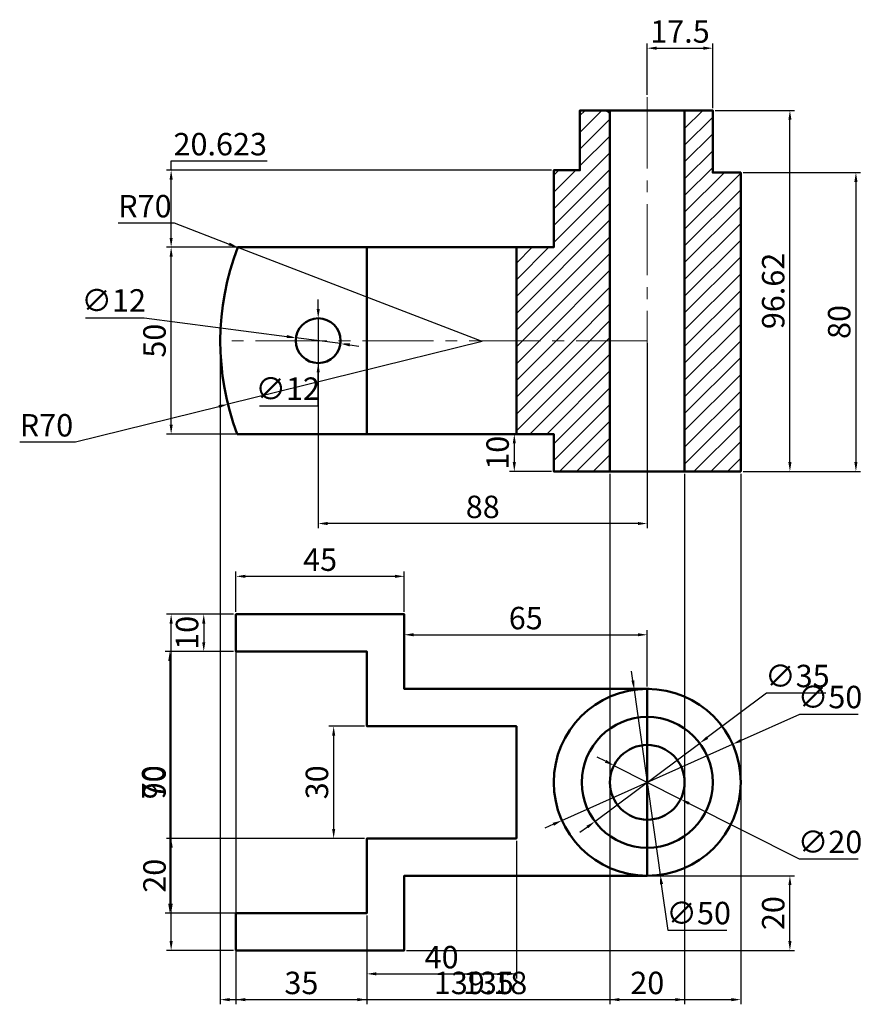
# Model space of a CAD drawing. Units: millimetres. Extents: x -19 to 206, y 5 to 269.
import ezdxf

# ---------------------------------------------------------------- set-up
doc = ezdxf.new("R2010")
doc.units = ezdxf.units.MM
doc.linetypes.add('CENTER2', pattern=[28.575, 19.05, -3.175, 3.175, -3.175])
for name, color, linetype, lineweight in [('M-CNTR', 4, 'CENTER2', 18), ('M-DIMS', 2, 'Continuous', 25), ('M-HATC', 8, 'Continuous', 18), ('M-OUTL', 7, 'Continuous', 50)]:
    doc.layers.add(name, color=color, linetype=linetype, lineweight=lineweight)
doc.styles.get("Standard").update_dxf_attribs({"font": 'arial.ttf'})
doc.dimstyles.new('ISO-25', dxfattribs={"dimtxt": 6, "dimasz": 2.5, "dimexe": 1.25, "dimexo": 0.625, "dimtad": 1, "dimtoh": 1, "dimdec": 0, "dimtxsty": 'Standard', "dimcen": 2.5, "dimadec": 0, "dimazin": 0, "dimtfac": 1, "dimtdec": 0, "dimtmove": 0, "dimatfit": 3, "dimfxl": 1, "dimarcsym": 0})

# ---------------------------------------------------------------- blocks, each defined once
blk = doc.blocks.new('*D1')
at = {"layer": 'Defpoints', "color": 0, "transparency": 16777216}
for p in [(54.94, 183.69), (66.84, 182.12)]:
    blk.add_point(p, dxfattribs=at)
at = {"layer": 'M-DIMS', "color": 0, "lineweight": -2, "transparency": 16777216}
for p, q in [((-1.34, 189.05), (14.35, 189.05)), ((14.35, 189.05), (52.46, 184.02)), ((66.84, 182.12), (54.94, 183.69)), ((69.31, 181.8), (71.79, 181.47))]:
    blk.add_line(p, q, dxfattribs=at)
at = {"layer": 'M-DIMS', "color": 0, "transparency": 16777216}
for points in [[(52.52, 184.43), (52.41, 183.61), (54.94, 183.69)], [(69.37, 182.21), (69.26, 181.38), (66.84, 182.12)]]:
    blk.add_solid(points, dxfattribs=at)
at = {"layer": 'M-DIMS', "color": 0, "transparency": 16777216, "insert": (6.19, 192.91), "char_height": 6, "attachment_point": 5}
blk.add_mtext('∅12', dxfattribs=at)
blk = doc.blocks.new('*D2')
at = {"layer": 'Defpoints', "color": 0, "transparency": 16777216}
for p in [(39.38, 207.88), (104.7, 182.73)]:
    blk.add_point(p, dxfattribs=at)
at = {"layer": 'M-DIMS', "color": 0, "lineweight": -2, "transparency": 16777216}
for p, q in [((7.38, 214.44), (22.32, 214.44)), ((22.32, 214.44), (37.04, 208.78)), ((104.7, 182.73), (39.38, 207.88))]:
    blk.add_line(p, q, dxfattribs=at)
at = {"layer": 'M-DIMS', "color": 0, "transparency": 16777216}
blk.add_solid([(37.19, 209.17), (36.89, 208.39), (39.38, 207.88)], dxfattribs=at)
at = {"layer": 'M-DIMS', "color": 0, "transparency": 16777216, "insert": (14.54, 218.13), "char_height": 6, "attachment_point": 5}
blk.add_mtext('R70', dxfattribs=at)
blk = doc.blocks.new('*D3')
at = {"layer": 'Defpoints', "color": 0, "transparency": 16777216}
for p in [(173.89, 227.91), (173.89, 147.91), (204.69, 147.91)]:
    blk.add_point(p, dxfattribs=at)
at = {"layer": 'M-DIMS', "color": 0, "lineweight": -2, "transparency": 16777216}
for p, q in [((174.51, 227.91), (205.94, 227.91)), ((204.69, 225.41), (204.69, 150.41)), ((174.51, 147.91), (205.94, 147.91))]:
    blk.add_line(p, q, dxfattribs=at)
at = {"layer": 'M-DIMS', "color": 0, "transparency": 16777216}
for points in [[(204.27, 225.41), (205.1, 225.41), (204.69, 227.91)], [(204.27, 150.41), (205.1, 150.41), (204.69, 147.91)]]:
    blk.add_solid(points, dxfattribs=at)
at = {"layer": 'M-DIMS', "color": 0, "transparency": 16777216, "insert": (201, 187.91), "char_height": 6, "attachment_point": 5, "rotation": 90}
blk.add_mtext('80', dxfattribs=at)
blk = doc.blocks.new('*D4')
at = {"layer": 'Defpoints', "color": 0, "transparency": 16777216}
for p in [(123.89, 157.91), (113.33, 147.91), (123.89, 147.91)]:
    blk.add_point(p, dxfattribs=at)
at = {"layer": 'M-DIMS', "color": 0, "lineweight": -2, "transparency": 16777216}
for p, q in [((123.26, 157.91), (112.08, 157.91)), ((113.33, 155.41), (113.33, 150.41)), ((123.26, 147.91), (112.08, 147.91))]:
    blk.add_line(p, q, dxfattribs=at)
at = {"layer": 'M-DIMS', "color": 0, "transparency": 16777216}
for points in [[(112.91, 155.41), (113.74, 155.41), (113.33, 157.91)], [(112.91, 150.41), (113.74, 150.41), (113.33, 147.91)]]:
    blk.add_solid(points, dxfattribs=at)
at = {"layer": 'M-DIMS', "color": 0, "transparency": 16777216, "insert": (109.64, 152.91), "char_height": 6, "attachment_point": 5, "rotation": 90}
blk.add_mtext('10', dxfattribs=at)
blk = doc.blocks.new('*D5')
at = {"layer": 'Defpoints', "color": 0, "transparency": 16777216}
for p in [(60.89, 182.91), (148.89, 182.91), (60.89, 133.98)]:
    blk.add_point(p, dxfattribs=at)
at = {"layer": 'M-DIMS', "color": 0, "lineweight": -2, "transparency": 16777216}
for p, q in [((60.89, 182.28), (60.89, 132.73)), ((148.89, 182.28), (148.89, 132.73)), ((146.39, 133.98), (63.39, 133.98))]:
    blk.add_line(p, q, dxfattribs=at)
at = {"layer": 'M-DIMS', "color": 0, "transparency": 16777216}
for points in [[(63.39, 134.39), (63.39, 133.56), (60.89, 133.98)], [(146.39, 134.39), (146.39, 133.56), (148.89, 133.98)]]:
    blk.add_solid(points, dxfattribs=at)
at = {"layer": 'M-DIMS', "color": 0, "transparency": 16777216, "insert": (104.89, 137.66), "char_height": 6, "attachment_point": 5}
blk.add_mtext('88', dxfattribs=at)
blk = doc.blocks.new('*D6')
at = {"layer": 'Defpoints', "color": 0, "transparency": 16777216}
for p in [(83.89, 119.85), (38.89, 109.72), (83.89, 109.72)]:
    blk.add_point(p, dxfattribs=at)
at = {"layer": 'M-DIMS', "color": 0, "lineweight": -2, "transparency": 16777216}
for p, q in [((38.89, 110.34), (38.89, 121.1)), ((41.39, 119.85), (81.39, 119.85)), ((83.89, 110.34), (83.89, 121.1))]:
    blk.add_line(p, q, dxfattribs=at)
at = {"layer": 'M-DIMS', "color": 0, "transparency": 16777216}
for points in [[(41.39, 120.27), (41.39, 119.43), (38.89, 119.85)], [(81.39, 120.27), (81.39, 119.43), (83.89, 119.85)]]:
    blk.add_solid(points, dxfattribs=at)
at = {"layer": 'M-DIMS', "color": 0, "transparency": 16777216, "insert": (61.39, 123.53), "char_height": 6, "attachment_point": 5}
blk.add_mtext('45', dxfattribs=at)
blk = doc.blocks.new('*D7')
at = {"layer": 'Defpoints', "color": 0, "transparency": 16777216}
for p in [(148.89, 104.21), (83.89, 89.72), (148.89, 89.72)]:
    blk.add_point(p, dxfattribs=at)
at = {"layer": 'M-DIMS', "color": 0, "lineweight": -2, "transparency": 16777216}
for p, q in [((83.89, 90.34), (83.89, 105.46)), ((148.89, 90.34), (148.89, 105.46)), ((86.39, 104.21), (146.39, 104.21))]:
    blk.add_line(p, q, dxfattribs=at)
at = {"layer": 'M-DIMS', "color": 0, "transparency": 16777216}
for points in [[(86.39, 104.63), (86.39, 103.8), (83.89, 104.21)], [(146.39, 104.63), (146.39, 103.8), (148.89, 104.21)]]:
    blk.add_solid(points, dxfattribs=at)
at = {"layer": 'M-DIMS', "color": 0, "transparency": 16777216, "insert": (116.39, 107.9), "char_height": 6, "attachment_point": 5}
blk.add_mtext('65', dxfattribs=at)
blk = doc.blocks.new('*D8')
at = {"layer": 'Defpoints', "color": 0, "transparency": 16777216}
for p in [(38.89, 109.72), (30.27, 99.72), (38.89, 99.72)]:
    blk.add_point(p, dxfattribs=at)
at = {"layer": 'M-DIMS', "color": 0, "lineweight": -2, "transparency": 16777216}
for p, q in [((38.26, 109.72), (29.02, 109.72)), ((30.27, 107.22), (30.27, 102.22)), ((38.26, 99.72), (29.02, 99.72))]:
    blk.add_line(p, q, dxfattribs=at)
at = {"layer": 'M-DIMS', "color": 0, "transparency": 16777216}
for points in [[(29.85, 107.22), (30.69, 107.22), (30.27, 109.72)], [(29.85, 102.22), (30.69, 102.22), (30.27, 99.72)]]:
    blk.add_solid(points, dxfattribs=at)
at = {"layer": 'M-DIMS', "color": 0, "transparency": 16777216, "insert": (26.58, 104.72), "char_height": 6, "attachment_point": 5, "rotation": 90}
blk.add_mtext('10', dxfattribs=at)
blk = doc.blocks.new('*D9')
at = {"layer": 'Defpoints', "color": 0, "transparency": 16777216}
for p in [(38.89, 99.72), (21.19, 29.72), (38.89, 29.72)]:
    blk.add_point(p, dxfattribs=at)
at = {"layer": 'M-DIMS', "color": 0, "lineweight": -2, "transparency": 16777216}
for p, q in [((38.26, 99.72), (19.94, 99.72)), ((21.19, 97.22), (21.19, 32.22)), ((38.26, 29.72), (19.94, 29.72))]:
    blk.add_line(p, q, dxfattribs=at)
at = {"layer": 'M-DIMS', "color": 0, "transparency": 16777216}
for points in [[(20.78, 97.22), (21.61, 97.22), (21.19, 99.72)], [(20.78, 32.22), (21.61, 32.22), (21.19, 29.72)]]:
    blk.add_solid(points, dxfattribs=at)
at = {"layer": 'M-DIMS', "color": 0, "transparency": 16777216, "insert": (17.5, 64.72), "char_height": 6, "attachment_point": 5, "rotation": 90}
blk.add_mtext('70', dxfattribs=at)
blk = doc.blocks.new('*D10')
at = {"layer": 'Defpoints', "color": 0, "transparency": 16777216}
for p in [(73.89, 79.72), (65.01, 49.72), (73.89, 49.72)]:
    blk.add_point(p, dxfattribs=at)
at = {"layer": 'M-DIMS', "color": 0, "lineweight": -2, "transparency": 16777216}
for p, q in [((73.26, 79.72), (63.76, 79.72)), ((65.01, 77.22), (65.01, 52.22)), ((73.26, 49.72), (63.76, 49.72))]:
    blk.add_line(p, q, dxfattribs=at)
at = {"layer": 'M-DIMS', "color": 0, "transparency": 16777216}
for points in [[(64.6, 77.22), (65.43, 77.22), (65.01, 79.72)], [(64.6, 52.22), (65.43, 52.22), (65.01, 49.72)]]:
    blk.add_solid(points, dxfattribs=at)
at = {"layer": 'M-DIMS', "color": 0, "transparency": 16777216, "insert": (61.32, 64.72), "char_height": 6, "attachment_point": 5, "rotation": 90}
blk.add_mtext('30', dxfattribs=at)
blk = doc.blocks.new('*D11')
at = {"layer": 'Defpoints', "color": 0, "transparency": 16777216}
for p in [(171.71, 74.92), (126.07, 54.52)]:
    blk.add_point(p, dxfattribs=at)
at = {"layer": 'M-DIMS', "color": 0, "lineweight": -2, "transparency": 16777216}
for p, q in [((189.59, 82.91), (173.99, 75.94)), ((205.31, 82.91), (189.59, 82.91)), ((126.07, 54.52), (171.71, 74.92)), ((123.78, 53.5), (121.5, 52.47))]:
    blk.add_line(p, q, dxfattribs=at)
at = {"layer": 'M-DIMS', "color": 0, "transparency": 16777216}
for points in [[(173.82, 76.32), (174.16, 75.56), (171.71, 74.92)], [(123.61, 53.88), (123.95, 53.11), (126.07, 54.52)]]:
    blk.add_solid(points, dxfattribs=at)
at = {"layer": 'M-DIMS', "color": 0, "transparency": 16777216, "insert": (197.76, 86.77), "char_height": 6, "attachment_point": 5}
blk.add_mtext('∅50', dxfattribs=at)
blk = doc.blocks.new('*D12')
at = {"layer": 'Defpoints', "color": 0, "transparency": 16777216}
for p in [(162.91, 75.18), (134.86, 54.25)]:
    blk.add_point(p, dxfattribs=at)
at = {"layer": 'M-DIMS', "color": 0, "lineweight": -2, "transparency": 16777216}
for p, q in [((180.82, 88.54), (164.92, 76.68)), ((196.61, 88.54), (180.82, 88.54)), ((134.86, 54.25), (162.91, 75.18)), ((132.86, 52.76), (130.85, 51.26))]:
    blk.add_line(p, q, dxfattribs=at)
at = {"layer": 'M-DIMS', "color": 0, "transparency": 16777216}
for points in [[(164.67, 77.01), (165.17, 76.35), (162.91, 75.18)], [(132.61, 53.09), (133.11, 52.43), (134.86, 54.25)]]:
    blk.add_solid(points, dxfattribs=at)
at = {"layer": 'M-DIMS', "color": 0, "transparency": 16777216, "insert": (189.03, 92.4), "char_height": 6, "attachment_point": 5}
blk.add_mtext('∅35', dxfattribs=at)
blk = doc.blocks.new('*D13')
at = {"layer": 'Defpoints', "color": 0, "transparency": 16777216}
for p in [(139.96, 69.23), (157.81, 60.21)]:
    blk.add_point(p, dxfattribs=at)
at = {"layer": 'M-DIMS', "color": 0, "lineweight": -2, "transparency": 16777216}
for p, q in [((137.73, 70.36), (135.5, 71.49)), ((139.96, 69.23), (157.81, 60.21)), ((189.59, 44.13), (160.04, 59.08)), ((205.31, 44.13), (189.59, 44.13))]:
    blk.add_line(p, q, dxfattribs=at)
at = {"layer": 'M-DIMS', "color": 0, "transparency": 16777216}
for points in [[(137.92, 70.73), (137.55, 69.99), (139.96, 69.23)], [(160.23, 59.45), (159.85, 58.71), (157.81, 60.21)]]:
    blk.add_solid(points, dxfattribs=at)
at = {"layer": 'M-DIMS', "color": 0, "transparency": 16777216, "insert": (197.76, 47.99), "char_height": 6, "attachment_point": 5}
blk.add_mtext('∅20', dxfattribs=at)
blk = doc.blocks.new('*D14')
at = {"layer": 'Defpoints', "color": 0, "transparency": 16777216}
for p in [(113.89, 49.72), (73.89, 29.72), (113.89, 13.47)]:
    blk.add_point(p, dxfattribs=at)
at = {"layer": 'M-DIMS', "color": 0, "lineweight": -2, "transparency": 16777216}
for p, q in [((113.89, 49.09), (113.89, 12.22)), ((73.89, 29.09), (73.89, 12.22)), ((76.39, 13.47), (111.39, 13.47))]:
    blk.add_line(p, q, dxfattribs=at)
at = {"layer": 'M-DIMS', "color": 0, "transparency": 16777216}
for points in [[(76.39, 13.89), (76.39, 13.06), (73.89, 13.47)], [(111.39, 13.89), (111.39, 13.06), (113.89, 13.47)]]:
    blk.add_solid(points, dxfattribs=at)
at = {"layer": 'M-DIMS', "color": 0, "transparency": 16777216, "insert": (93.89, 17.16), "char_height": 6, "attachment_point": 5}
blk.add_mtext('40', dxfattribs=at)
blk = doc.blocks.new('*D15')
at = {"layer": 'Defpoints', "color": 0, "transparency": 16777216}
for p in [(166.39, 261.18), (148.89, 248.03), (166.39, 244.53)]:
    blk.add_point(p, dxfattribs=at)
at = {"layer": 'M-DIMS', "color": 0, "lineweight": -2, "transparency": 16777216}
for p, q in [((148.89, 248.66), (148.89, 262.43)), ((151.39, 261.18), (163.89, 261.18)), ((166.39, 245.16), (166.39, 262.43))]:
    blk.add_line(p, q, dxfattribs=at)
at = {"layer": 'M-DIMS', "color": 0, "transparency": 16777216}
for points in [[(151.39, 261.6), (151.39, 260.76), (148.89, 261.18)], [(163.89, 261.6), (163.89, 260.76), (166.39, 261.18)]]:
    blk.add_solid(points, dxfattribs=at)
at = {"layer": 'M-DIMS', "color": 0, "transparency": 16777216, "insert": (157.64, 264.87), "char_height": 6, "attachment_point": 5}
blk.add_mtext('17.5', dxfattribs=at)
blk = doc.blocks.new('*D16')
at = {"layer": 'Defpoints', "color": 0, "transparency": 16777216}
for p in [(138.89, 147.91), (158.89, 147.91), (158.89, 6.57)]:
    blk.add_point(p, dxfattribs=at)
at = {"layer": 'M-DIMS', "color": 0, "lineweight": -2, "transparency": 16777216}
for p, q in [((138.89, 147.28), (138.89, 5.32)), ((158.89, 147.28), (158.89, 5.32)), ((141.39, 6.57), (156.39, 6.57))]:
    blk.add_line(p, q, dxfattribs=at)
at = {"layer": 'M-DIMS', "color": 0, "transparency": 16777216}
for points in [[(141.39, 6.99), (141.39, 6.15), (138.89, 6.57)], [(156.39, 6.99), (156.39, 6.15), (158.89, 6.57)]]:
    blk.add_solid(points, dxfattribs=at)
at = {"layer": 'M-DIMS', "color": 0, "transparency": 16777216, "insert": (148.89, 10.26), "char_height": 6, "attachment_point": 5}
blk.add_mtext('20', dxfattribs=at)
blk = doc.blocks.new('*D17')
at = {"layer": 'Defpoints', "color": 0, "transparency": 16777216}
for p in [(73.89, 29.72), (38.89, 19.72), (73.89, 6.57)]:
    blk.add_point(p, dxfattribs=at)
at = {"layer": 'M-DIMS', "color": 0, "lineweight": -2, "transparency": 16777216}
for p, q in [((73.89, 29.09), (73.89, 5.32)), ((38.89, 19.09), (38.89, 5.32)), ((41.39, 6.57), (71.39, 6.57))]:
    blk.add_line(p, q, dxfattribs=at)
at = {"layer": 'M-DIMS', "color": 0, "transparency": 16777216}
for points in [[(41.39, 6.99), (41.39, 6.15), (38.89, 6.57)], [(71.39, 6.99), (71.39, 6.15), (73.89, 6.57)]]:
    blk.add_solid(points, dxfattribs=at)
at = {"layer": 'M-DIMS', "color": 0, "transparency": 16777216, "insert": (56.39, 10.26), "char_height": 6, "attachment_point": 5}
blk.add_mtext('35', dxfattribs=at)
blk = doc.blocks.new('*D18')
at = {"layer": 'Defpoints', "color": 0, "transparency": 16777216}
for p in [(21.55, 109.72), (38.89, 109.72), (38.89, 19.72)]:
    blk.add_point(p, dxfattribs=at)
at = {"layer": 'M-DIMS', "color": 0, "lineweight": -2, "transparency": 16777216}
for p, q in [((38.26, 109.72), (20.3, 109.72)), ((21.55, 22.22), (21.55, 107.22)), ((38.26, 19.72), (20.3, 19.72))]:
    blk.add_line(p, q, dxfattribs=at)
at = {"layer": 'M-DIMS', "color": 0, "transparency": 16777216}
for points in [[(21.14, 107.22), (21.97, 107.22), (21.55, 109.72)], [(21.14, 22.22), (21.97, 22.22), (21.55, 19.72)]]:
    blk.add_solid(points, dxfattribs=at)
at = {"layer": 'M-DIMS', "color": 0, "transparency": 16777216, "insert": (17.87, 64.72), "char_height": 6, "attachment_point": 5, "rotation": 90}
blk.add_mtext('90', dxfattribs=at)
blk = doc.blocks.new('*D19')
at = {"layer": 'Defpoints', "color": 0, "transparency": 16777216}
for p in [(34.7, 182.92), (173.89, 147.91), (173.89, 6.57)]:
    blk.add_point(p, dxfattribs=at)
at = {"layer": 'M-DIMS', "color": 0, "lineweight": -2, "transparency": 16777216}
for p, q in [((34.7, 182.3), (34.7, 5.32)), ((173.89, 147.28), (173.89, 5.32)), ((37.2, 6.57), (171.39, 6.57))]:
    blk.add_line(p, q, dxfattribs=at)
at = {"layer": 'M-DIMS', "color": 0, "transparency": 16777216}
for points in [[(37.2, 6.99), (37.2, 6.15), (34.7, 6.57)], [(171.39, 6.99), (171.39, 6.15), (173.89, 6.57)]]:
    blk.add_solid(points, dxfattribs=at)
at = {"layer": 'M-DIMS', "color": 0, "transparency": 16777216, "insert": (104.3, 10.26), "char_height": 6, "attachment_point": 5}
blk.add_mtext('139.18', dxfattribs=at)
blk = doc.blocks.new('*D20')
at = {"layer": 'Defpoints', "color": 0, "transparency": 16777216}
for p in [(166.39, 244.53), (187.04, 244.53), (173.89, 147.91)]:
    blk.add_point(p, dxfattribs=at)
at = {"layer": 'M-DIMS', "color": 0, "lineweight": -2, "transparency": 16777216}
for p, q in [((167.01, 244.53), (188.29, 244.53)), ((187.04, 150.41), (187.04, 242.03)), ((174.51, 147.91), (188.29, 147.91))]:
    blk.add_line(p, q, dxfattribs=at)
at = {"layer": 'M-DIMS', "color": 0, "transparency": 16777216}
for points in [[(186.62, 242.03), (187.45, 242.03), (187.04, 244.53)], [(186.62, 150.41), (187.45, 150.41), (187.04, 147.91)]]:
    blk.add_solid(points, dxfattribs=at)
at = {"layer": 'M-DIMS', "color": 0, "transparency": 16777216, "insert": (183.35, 196.22), "char_height": 6, "attachment_point": 5, "rotation": 90}
blk.add_mtext('96.62', dxfattribs=at)
blk = doc.blocks.new('*D21')
at = {"layer": 'Defpoints', "color": 0, "transparency": 16777216}
for p in [(21.55, 207.91), (123.89, 207.91), (123.89, 157.91)]:
    blk.add_point(p, dxfattribs=at)
at = {"layer": 'M-DIMS', "color": 0, "lineweight": -2, "transparency": 16777216}
for p, q in [((123.26, 207.91), (20.3, 207.91)), ((21.55, 160.41), (21.55, 205.41)), ((123.26, 157.91), (20.3, 157.91))]:
    blk.add_line(p, q, dxfattribs=at)
at = {"layer": 'M-DIMS', "color": 0, "transparency": 16777216}
for points in [[(21.14, 205.41), (21.97, 205.41), (21.55, 207.91)], [(21.14, 160.41), (21.97, 160.41), (21.55, 157.91)]]:
    blk.add_solid(points, dxfattribs=at)
at = {"layer": 'M-DIMS', "color": 0, "transparency": 16777216, "insert": (17.87, 182.91), "char_height": 6, "attachment_point": 5, "rotation": 90}
blk.add_mtext('50', dxfattribs=at)
blk = doc.blocks.new('*D22')
at = {"layer": 'Defpoints', "color": 0, "transparency": 16777216}
for p in [(173.89, 147.91), (38.89, 109.72), (173.89, 6.57)]:
    blk.add_point(p, dxfattribs=at)
at = {"layer": 'M-DIMS', "color": 0, "lineweight": -2, "transparency": 16777216}
for p, q in [((173.89, 147.28), (173.89, 5.32)), ((38.89, 109.09), (38.89, 5.32)), ((41.39, 6.57), (171.39, 6.57))]:
    blk.add_line(p, q, dxfattribs=at)
at = {"layer": 'M-DIMS', "color": 0, "transparency": 16777216}
for points in [[(41.39, 6.99), (41.39, 6.15), (38.89, 6.57)], [(171.39, 6.99), (171.39, 6.15), (173.89, 6.57)]]:
    blk.add_solid(points, dxfattribs=at)
at = {"layer": 'M-DIMS', "color": 0, "transparency": 16777216, "insert": (106.39, 10.26), "char_height": 6, "attachment_point": 5}
blk.add_mtext('135', dxfattribs=at)
blk = doc.blocks.new('*D23')
at = {"layer": 'Defpoints', "color": 0, "transparency": 16777216}
for p in [(21.55, 49.72), (73.89, 49.72), (73.89, 29.72)]:
    blk.add_point(p, dxfattribs=at)
at = {"layer": 'M-DIMS', "color": 0, "lineweight": -2, "transparency": 16777216}
for p, q in [((73.26, 49.72), (20.3, 49.72)), ((21.55, 32.22), (21.55, 47.22)), ((73.26, 29.72), (20.3, 29.72))]:
    blk.add_line(p, q, dxfattribs=at)
at = {"layer": 'M-DIMS', "color": 0, "transparency": 16777216}
for points in [[(21.14, 47.22), (21.97, 47.22), (21.55, 49.72)], [(21.14, 32.22), (21.97, 32.22), (21.55, 29.72)]]:
    blk.add_solid(points, dxfattribs=at)
at = {"layer": 'M-DIMS', "color": 0, "transparency": 16777216, "insert": (17.87, 39.72), "char_height": 6, "attachment_point": 5, "rotation": 90}
blk.add_mtext('20', dxfattribs=at)
blk = doc.blocks.new('*D24')
at = {"layer": 'Defpoints', "color": 0, "transparency": 16777216}
for p in [(83.89, 39.72), (187.04, 39.72), (83.89, 19.72)]:
    blk.add_point(p, dxfattribs=at)
at = {"layer": 'M-DIMS', "color": 0, "lineweight": -2, "transparency": 16777216}
for p, q in [((84.51, 39.72), (188.29, 39.72)), ((187.04, 22.22), (187.04, 37.22)), ((84.51, 19.72), (188.29, 19.72))]:
    blk.add_line(p, q, dxfattribs=at)
at = {"layer": 'M-DIMS', "color": 0, "transparency": 16777216}
for points in [[(186.62, 37.22), (187.45, 37.22), (187.04, 39.72)], [(186.62, 22.22), (187.45, 22.22), (187.04, 19.72)]]:
    blk.add_solid(points, dxfattribs=at)
at = {"layer": 'M-DIMS', "color": 0, "transparency": 16777216, "insert": (183.35, 29.72), "char_height": 6, "attachment_point": 5, "rotation": 90}
blk.add_mtext('20', dxfattribs=at)
blk = doc.blocks.new('*D25')
at = {"layer": 'Defpoints', "color": 0, "transparency": 16777216}
for p in [(21.55, 228.53), (123.89, 228.53), (123.89, 207.91)]:
    blk.add_point(p, dxfattribs=at)
at = {"layer": 'M-DIMS', "color": 0, "lineweight": -2, "transparency": 16777216}
for p, q in [((21.55, 228.53), (21.55, 231.03)), ((21.55, 231.03), (47.19, 231.03)), ((123.26, 228.53), (20.3, 228.53)), ((21.55, 210.41), (21.55, 226.03)), ((123.26, 207.91), (20.3, 207.91))]:
    blk.add_line(p, q, dxfattribs=at)
at = {"layer": 'M-DIMS', "color": 0, "transparency": 16777216}
for points in [[(21.14, 226.03), (21.97, 226.03), (21.55, 228.53)], [(21.14, 210.41), (21.97, 210.41), (21.55, 207.91)]]:
    blk.add_solid(points, dxfattribs=at)
at = {"layer": 'M-DIMS', "color": 0, "transparency": 16777216, "insert": (34.68, 234.72), "char_height": 6, "attachment_point": 5}
blk.add_mtext('20.623', dxfattribs=at)
blk = doc.blocks.new('*D26')
at = {"layer": 'Defpoints', "color": 0, "transparency": 16777216}
for p in [(145.41, 89.48), (152.37, 39.96)]:
    blk.add_point(p, dxfattribs=at)
at = {"layer": 'M-DIMS', "color": 0, "lineweight": -2, "transparency": 16777216}
for p, q in [((145.06, 91.95), (144.71, 94.43)), ((145.41, 89.48), (152.37, 39.96)), ((154.45, 25.11), (152.71, 37.49)), ((170.18, 25.11), (154.45, 25.11))]:
    blk.add_line(p, q, dxfattribs=at)
at = {"layer": 'M-DIMS', "color": 0, "transparency": 16777216}
for points in [[(145.47, 92.01), (144.65, 91.89), (145.41, 89.48)], [(153.13, 37.54), (152.3, 37.43), (152.37, 39.96)]]:
    blk.add_solid(points, dxfattribs=at)
at = {"layer": 'M-DIMS', "color": 0, "transparency": 16777216, "insert": (162.63, 28.96), "char_height": 6, "attachment_point": 5}
blk.add_mtext('∅50', dxfattribs=at)
blk = doc.blocks.new('*D27')
at = {"layer": 'Defpoints', "color": 0, "transparency": 16777216}
for p in [(60.89, 188.91), (60.89, 176.91)]:
    blk.add_point(p, dxfattribs=at)
at = {"layer": 'M-DIMS', "color": 0, "lineweight": -2, "transparency": 16777216}
for p, q in [((60.89, 191.41), (60.89, 193.91)), ((60.89, 188.91), (60.89, 176.91)), ((60.89, 165.45), (60.89, 174.41)), ((45.2, 165.45), (60.89, 165.45))]:
    blk.add_line(p, q, dxfattribs=at)
at = {"layer": 'M-DIMS', "color": 0, "transparency": 16777216}
for points in [[(60.47, 191.41), (61.3, 191.41), (60.89, 188.91)], [(60.47, 174.41), (61.3, 174.41), (60.89, 176.91)]]:
    blk.add_solid(points, dxfattribs=at)
at = {"layer": 'M-DIMS', "color": 0, "transparency": 16777216, "insert": (52.73, 169.3), "char_height": 6, "attachment_point": 5}
blk.add_mtext('∅12', dxfattribs=at)
blk = doc.blocks.new('*D28')
at = {"layer": 'Defpoints', "color": 0, "transparency": 16777216}
for p in [(104.7, 182.73), (36.76, 165.9)]:
    blk.add_point(p, dxfattribs=at)
at = {"layer": 'M-DIMS', "color": 0, "lineweight": -2, "transparency": 16777216}
for p, q in [((104.7, 182.73), (36.76, 165.9)), ((-4.01, 155.8), (34.33, 165.3)), ((-18.95, 155.8), (-4.01, 155.8))]:
    blk.add_line(p, q, dxfattribs=at)
at = {"layer": 'M-DIMS', "color": 0, "transparency": 16777216}
blk.add_solid([(34.23, 165.7), (34.43, 164.89), (36.76, 165.9)], dxfattribs=at)
at = {"layer": 'M-DIMS', "color": 0, "transparency": 16777216, "insert": (-11.79, 159.49), "char_height": 6, "attachment_point": 5}
blk.add_mtext('R70', dxfattribs=at)

msp = doc.modelspace()

# ---------------------------------------------------------------- hatches: boundary and pattern name
at = {"layer": 'M-HATC'}
h = msp.add_hatch(dxfattribs=at)
h.set_pattern_fill('ANSI31', color=256)
h.paths.add_polyline_path([(138.8881, 243.9555, 0.00426516), (137.8416, 244.5309), (130.8881, 244.5309), (130.8881, 228.5309), (123.8881, 228.5309), (123.8881, 207.9077), (113.8881, 207.9077), (113.8881, 182.9077), (138.8881, 182.9077)])
h = msp.add_hatch(dxfattribs=at)
h.set_pattern_fill('ANSI31', color=256)
h.paths.add_polyline_path([(138.8881, 182.9077), (113.8881, 182.9077), (113.8881, 157.9077), (123.8881, 157.9077), (123.8881, 147.9077), (138.8881, 147.9077)])
h.paths.add_polyline_path([(173.8881, 227.9077), (166.3881, 227.9077), (166.3881, 244.5309), (158.8881, 244.5309), (158.8881, 147.9077), (173.8881, 147.9077)])

# ---------------------------------------------------------------- linework, layer by layer
at = {"layer": 'M-CNTR'}
for p, q in [((148.8881, 248.0309), (148.8881, 144.7193)), ((148.8881, 182.9077), (36.1381, 182.9077)), ((60.8881, 170.7657), (60.8881, 182.9077))]:
    msp.add_line(p, q, dxfattribs=at)
at = {"layer": 'M-OUTL'}
for p, q in [((138.8881, 244.5309), (138.8881, 147.9077)), ((158.8881, 147.9077), (158.8881, 244.5309)), ((73.8881, 157.9077), (73.8881, 207.9077)), ((113.8881, 157.9077), (113.8881, 207.9077))]:
    msp.add_line(p, q, dxfattribs=at)
msp.add_lwpolyline([(39.253, 157.9077, -0.18466136), (39.3881, 207.9077), (123.8881, 207.9077), (123.8881, 228.5309), (130.8881, 228.5309), (130.8881, 244.5309), (138.8881, 244.5309), (138.8881, 244.5309), (158.8881, 244.5309), (166.3881, 244.5309), (166.3881, 227.9077), (173.8881, 227.9077), (173.8881, 147.9077), (123.8881, 147.9077), (123.8881, 157.9077), (39.8881, 157.9077)], format="xyb", close=True, dxfattribs=at)
msp.add_lwpolyline([(148.8881, 89.7193), (148.8881, 39.7193), (83.8881, 39.7193), (83.8881, 19.7193), (38.8881, 19.7193), (38.8881, 29.7193), (73.8881, 29.7193), (73.8881, 49.7193), (113.8881, 49.7193), (113.8881, 79.7193), (73.8881, 79.7193), (73.8881, 99.7193), (38.8881, 99.7193), (38.8881, 109.7193), (83.8881, 109.7193), (83.8881, 89.7193), (149.4084, 89.7193)], dxfattribs=at)
for centre, radius in [((60.8881, 182.9077), 6), ((148.8881, 64.7193), 25), ((148.8881, 64.7193), 17.5), ((148.8881, 64.7193), 10)]:
    msp.add_circle(centre, radius, dxfattribs=at)
msp.add_arc((104.6365, 182.9077), 70, 60.704855, 61.682353, dxfattribs=at)

# ---------------------------------------------------------------- dimensions: what is measured, and where the dimension line sits
at = {"layer": 'M-DIMS'}
for base, p1, p2, override, picture, middle in [((166.3881, 261.1809), (148.8881, 248.0309), (166.3881, 244.5309), {"dimdec": 1, "dimlfac": 1, "dimrnd": 0, "dimzin": 0, "dimdsep": 46, "dimlunit": 2}, '*D15', (157.6381, 264.8693)), ((173.8881, 6.5693), (34.704, 182.9202), (173.8881, 147.9077), {"dimdec": 2, "dimlfac": 1, "dimrnd": 0, "dimzin": 0, "dimdsep": 46, "dimlunit": 2}, '*D19', (104.296, 10.2598)), ((60.8881, 133.9751), (148.8881, 182.9077), (60.8881, 182.9077), {"dimclrd": 0, "dimclre": 0, "dimclrt": 0}, '*D5', (104.8881, 137.6635)), ((173.8881, 6.5693), (38.8881, 109.7193), (173.8881, 147.9077), {"dimdec": 0, "dimlfac": 1, "dimrnd": 0, "dimzin": 0, "dimdsep": 46, "dimlunit": 2}, '*D22', (106.3881, 10.2598)), ((158.8881, 6.5693), (138.8881, 147.9077), (158.8881, 147.9077), {"dimdec": 0, "dimlfac": 1, "dimrnd": 0, "dimzin": 0, "dimdsep": 46, "dimlunit": 2}, '*D16', (148.8881, 10.2577)), ((83.8881, 119.8514), (38.8881, 109.7193), (83.8881, 109.7193), {"dimclrd": 0, "dimclre": 0, "dimclrt": 0}, '*D6', (61.3881, 123.5276)), ((148.8881, 104.2142), (83.8881, 89.7193), (148.8881, 89.7193), {"dimclrd": 0, "dimclre": 0, "dimclrt": 0}, '*D7', (116.3881, 107.9026)), ((113.8881, 13.4727), (73.8881, 29.7193), (113.8881, 49.7193), {"dimclrd": 0, "dimclre": 0, "dimclrt": 0}, '*D14', (93.8881, 17.1612)), ((73.8881, 6.5693), (38.8881, 19.7193), (73.8881, 29.7193), {"dimdec": 0, "dimlfac": 1, "dimrnd": 0, "dimzin": 0, "dimdsep": 46, "dimlunit": 2}, '*D17', (56.3881, 10.2598))]:
    dim = msp.add_linear_dim(base=base, p1=p1, p2=p2, dimstyle='ISO-25', override=override, dxfattribs=at)
    dim.commit()
    dim.dimension.update_dxf_attribs({"geometry": picture, "text_midpoint": middle})
for base, p1, p2, override, picture, middle in [((187.0381, 244.5309), (173.8881, 147.9077), (166.3881, 244.5309), {"dimdec": 2, "dimlfac": 1, "dimrnd": 0, "dimzin": 0, "dimdsep": 46, "dimlunit": 2}, '*D20', (183.3496, 196.2193)), ((21.554, 228.5309), (123.8881, 207.9077), (123.8881, 228.5309), {"dimdec": 3, "dimlfac": 1, "dimrnd": 0, "dimzin": 0, "dimdsep": 46, "dimlunit": 2}, '*D25', (34.6844, 234.7214)), ((204.6852, 147.9077), (173.8881, 227.9077), (173.8881, 147.9077), {"dimclrd": 0, "dimclre": 0, "dimclrt": 0}, '*D3', (200.9967, 187.9077)), ((21.554, 207.9077), (123.8881, 157.9077), (123.8881, 207.9077), {"dimdec": 0, "dimlfac": 1, "dimrnd": 0, "dimzin": 0, "dimdsep": 46, "dimlunit": 2}, '*D21', (17.8655, 182.9077)), ((113.3279, 147.9077), (123.8881, 157.9077), (123.8881, 147.9077), {"dimclrd": 0, "dimclre": 0, "dimclrt": 0}, '*D4', (109.6395, 152.9077)), ((21.554, 109.7193), (38.8881, 19.7193), (38.8881, 109.7193), {"dimdec": 0, "dimlfac": 1, "dimrnd": 0, "dimzin": 0, "dimdsep": 46, "dimlunit": 2}, '*D18', (17.8655, 64.7193)), ((30.2689, 99.7193), (38.8881, 109.7193), (38.8881, 99.7193), {"dimclrd": 0, "dimclre": 0, "dimclrt": 0}, '*D8', (26.5805, 104.7193)), ((21.192, 29.7193), (38.8881, 99.7193), (38.8881, 29.7193), {"dimclrd": 0, "dimclre": 0, "dimclrt": 0}, '*D9', (17.5035, 64.7193)), ((65.0117, 49.7193), (73.8881, 79.7193), (73.8881, 49.7193), {"dimclrd": 0, "dimclre": 0, "dimclrt": 0}, '*D10', (61.3213, 64.7193)), ((21.554, 49.7193), (73.8881, 29.7193), (73.8881, 49.7193), {"dimdec": 0, "dimlfac": 1, "dimrnd": 0, "dimzin": 0, "dimdsep": 46, "dimlunit": 2}, '*D23', (17.8655, 39.7193)), ((187.0381, 39.7193), (83.8881, 19.7193), (83.8881, 39.7193), {"dimdec": 0, "dimlfac": 1, "dimrnd": 0, "dimzin": 0, "dimdsep": 46, "dimlunit": 2}, '*D24', (183.3496, 29.7193))]:
    dim = msp.add_linear_dim(base=base, p1=p1, p2=p2, angle=90, dimstyle='ISO-25', override=override, dxfattribs=at)
    dim.commit()
    dim.dimension.update_dxf_attribs({"geometry": picture, "text_midpoint": middle})
for mpoint, override, picture, middle in [((39.3767, 207.8781), {"dimclrd": 0, "dimclre": 0, "dimclrt": 0}, '*D2', (14.5392, 214.443)), ((36.7579, 165.8976), {"dimdec": 0, "dimlfac": 1, "dimrnd": 0, "dimzin": 0, "dimdsep": 46, "dimlunit": 2}, '*D28', (-4.0096, 155.7975))]:
    dim = msp.add_radius_dim(center=(104.7037, 182.7311), mpoint=mpoint, dimstyle='ISO-25', override=override, dxfattribs=at)
    dim.commit()
    dim.dimension.update_dxf_attribs({"geometry": picture, "text_midpoint": middle, "dimtype": 164})
for p1, p2, override, picture, middle in [((66.8364, 182.1223), (54.9397, 183.6931), {"dimclrd": 0, "dimclre": 0, "dimclrt": 0}, '*D1', (14.3503, 189.0524)), ((60.8881, 188.9077), (60.888, 176.9077), {"dimdec": 0, "dimlfac": 1, "dimrnd": 0, "dimzin": 0, "dimdsep": 46, "dimlunit": 2}, '*D27', (52.7322, 165.4452)), ((134.8617, 54.2545), (162.9144, 75.1841), {"dimclrd": 0, "dimclre": 0, "dimclrt": 0}, '*D12', (189.0301, 88.5439)), ((145.4092, 89.4761), (152.3669, 39.9625), {"dimdec": 0, "dimlfac": 1, "dimrnd": 0, "dimzin": 0, "dimdsep": 46, "dimlunit": 2}, '*D26', (162.6304, 25.1085)), ((126.0652, 54.5155), (171.7109, 74.9232), {"dimclrd": 0, "dimclre": 0, "dimclrt": 0}, '*D11', (197.7613, 82.9145)), ((139.9646, 69.2329), (157.8115, 60.2057), {"dimclrd": 0, "dimclre": 0, "dimclrt": 0}, '*D13', (197.7613, 44.1342))]:
    dim = msp.add_diameter_dim_2p(p1=p1, p2=p2, dimstyle='ISO-25', override=override, dxfattribs=at)
    dim.commit()
    dim.dimension.update_dxf_attribs({"geometry": picture, "text_midpoint": middle, "dimtype": 163})

doc.saveas('drawing.dxf')
